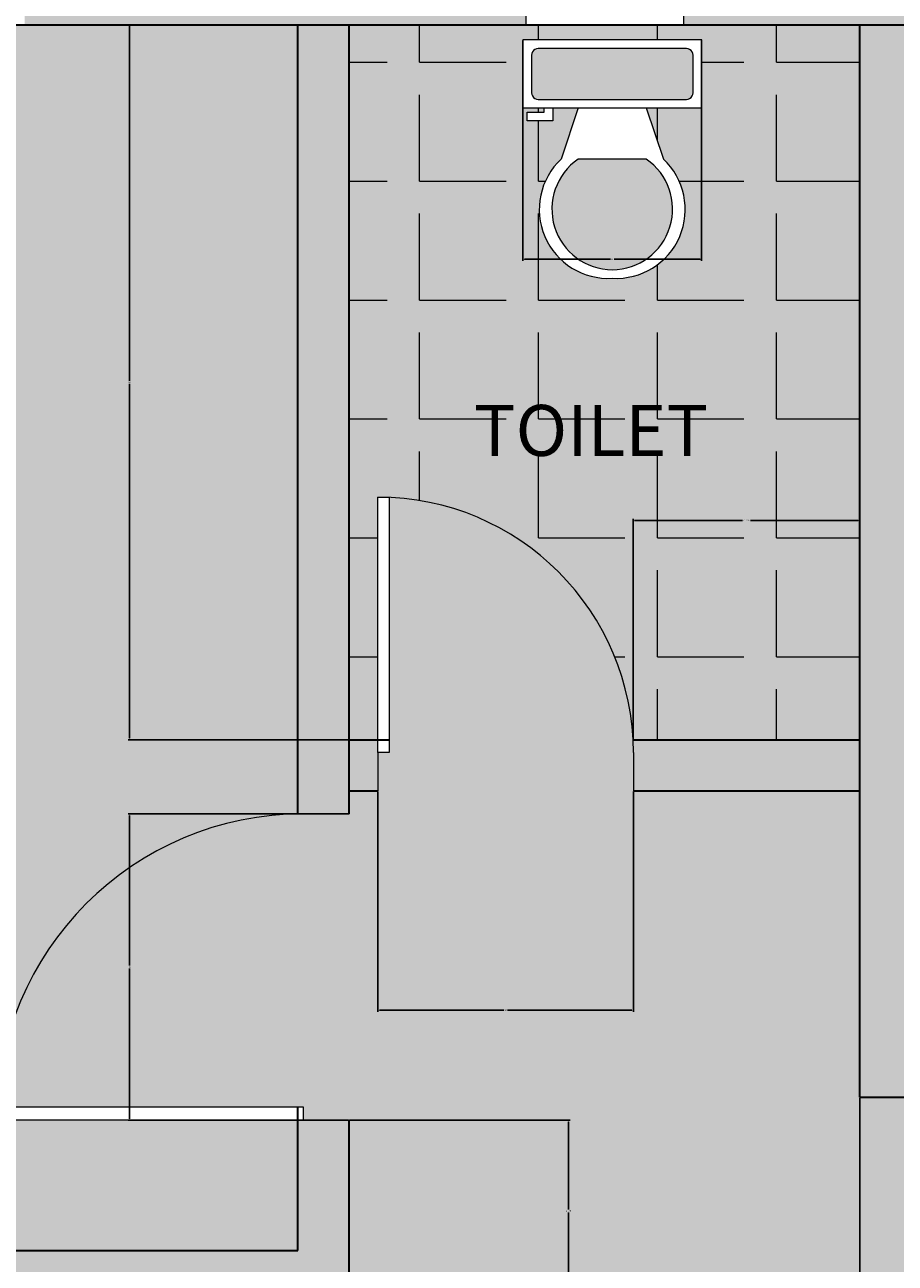
# Model space of a CAD drawing. Units: inches. Extents: x 3024 to 3952, y 1308 to 1863.
# Tile 23 of 29: x 3195 to 3297, y 1633 to 1779. Entities that reach past the tile are written whole.
import ezdxf

# ---------------------------------------------------------------- set-up
doc = ezdxf.new("R2010")
doc.units = ezdxf.units.IN
for name, color, linetype, lineweight in [('A-ANNO-DIMS', 2, 'Continuous', 18), ('A-AREA-IDEN', 7, 'Continuous', 18), ('A-DOOR', 4, 'Continuous', 18), ('A-FLOR-FIXT', 9, 'Continuous', 18), ('A-FLOR-FIXT-PATT', 7, 'Continuous', 13), ('A-FLOR-TILE-PATT', 7, 'Continuous', 13), ('A-GLAZ', 4, 'Continuous', 18), ('A-WALL', 7, 'Continuous', 35)]:
    doc.layers.add(name, color=color, linetype=linetype, lineweight=lineweight)
doc.layers.add('A-FLOR-PATT', color=254, linetype='Continuous', lineweight=13, true_color=0xfeeab9)
doc.layers.add('A-WALL-PATT', color=254, linetype='Continuous', lineweight=13, true_color=0xcecce6)
doc.styles.get("Standard").update_dxf_attribs({"font": 'arial.ttf'})
doc.dimstyles.get("Standard").update_dxf_attribs({"dimtxt": 0.18, "dimasz": 0.18, "dimexe": 0.18, "dimexo": 0.0625, "dimgap": 0.09, "dimtad": 0, "dimtih": 1, "dimtoh": 1, "dimdec": 4, "dimzin": 0, "dimdsep": 46, "dimtxsty": 'Standard', "dimcen": 0.09, "dimadec": 0, "dimazin": 0, "dimtfac": 1, "dimtdec": 4, "dimtofl": 0, "dimtmove": 0, "dimatfit": 3, "dimfxl": 1, "dimtolj": 1, "dimtzin": 0, "dimarcsym": 0})

# ---------------------------------------------------------------- blocks, each defined once
blk = doc.blocks.new('*U2')
for p, q in [((0, 0), (0, -6)), ((40, 0), (40, -6))]:
    blk.add_line(p, q)
blk.add_lwpolyline([(0, 0), (0, 40), (1.75, 40), (1.75, 0)], close=True)
blk.add_arc((0, 0), 40, 0, 90)
blk = doc.blocks.new('*U4')
for p, q in [((-40, 0), (-40, 6)), ((0, 0), (0, 6))]:
    blk.add_line(p, q)
blk.add_lwpolyline([(0, 0), (0, -40), (-1.75, -40), (-1.75, 0)], close=True)
blk.add_arc((0, 0), 40, 180, 270)
blk = doc.blocks.new('*U12')
for p, q in [((9.5, -6), (9.5, -2)), ((-10, -8.5), (-8, -8.5)), ((-10, -9.5), (-10, -8.5)), ((-8, -8.5), (-8, -8)), ((-7, -8), (-7, -9.5)), ((-4, -8), (-6, -14)), ((4, -8), (6, -14)), ((-7, -9.5), (-10, -9.5)), ((4, -14), (-4, -14))]:
    blk.add_line(p, q)
blk.add_lwpolyline([(10.5, -8), (10.5, 0), (-10.5, 0), (-10.5, -8)], close=True)
for points in [[(8.5, -1), (-8.5, -1)], [(-9.5, -2), (-9.5, -6)], [(-8.5, -7), (8.5, -7)]]:
    blk.add_lwpolyline(points)
for centre, radius, start, end in [((-8.625, -1.875), 0.8839, 81.8699, 188.1301), ((8.625, -1.875), 0.8839, 351.8699, 98.1301), ((-8.625, -6.125), 0.8839, 171.869898, 278.1301), ((8.625, -6.125), 0.8839, 261.8699, 8.1301), ((-0.4772, -19.9188), 8.0953, 133.01722, 273.38), ((0.0374, -19.8731), 7.127, 124.50543, 269.7), ((-0.0373, -19.8731), 7.127, 270.3, 55.4946), ((0.4773, -19.9188), 8.0953, 266.62, 46.9828)]:
    blk.add_arc(centre, radius, start, end)
blk = doc.blocks.new('WIN-BATH-18p5IN')
for p, q in [((0, 5.99), (0, 9)), ((18.52, 6.41), (18.52, 9)), ((18.52, 6.41), (18.52, 5.99)), ((0, 3.28), (0, 0)), ((18.52, 3.69), (18.52, 0))]:
    blk.add_line(p, q)
blk.add_lwpolyline([(0, 5.99), (18.52, 5.99), (18.52, 3.28), (0, 3.28)], close=True)
blk = doc.blocks.new('*D51')
at = {"layer": 'A-ANNO-DIMS', "color": 0, "lineweight": -2, "transparency": 16777216}
for p, q in [((3232.7, 1778.61), (3206.81, 1778.61)), ((3206.99, 1778.43), (3206.99, 1736.79)), ((3206.99, 1694.79), (3206.99, 1736.42)), ((3232.7, 1694.61), (3206.81, 1694.61))]:
    blk.add_line(p, q, dxfattribs=at)
at = {"layer": 'A-ANNO-DIMS', "color": 0, "transparency": 16777216}
for points in [[(3206.96, 1778.43), (3207.02, 1778.43), (3206.99, 1778.61)], [(3206.96, 1694.79), (3207.02, 1694.79), (3206.99, 1694.61)]]:
    blk.add_solid(points, dxfattribs=at)
at = {"layer": 'Defpoints', "color": 0, "transparency": 16777216}
for p in [(3206.99, 1778.61), (3232.76, 1778.61), (3232.76, 1694.61)]:
    blk.add_point(p, dxfattribs=at)
at = {"layer": 'A-ANNO-DIMS', "color": 0, "transparency": 16777216, "insert": (3206.99, 1736.61), "char_height": 0.18, "attachment_point": 5}
blk.add_mtext('\\A1;84', dxfattribs=at)
blk = doc.blocks.new('*D56')
at = {"layer": 'A-ANNO-DIMS', "color": 0, "lineweight": -2, "transparency": 16777216}
for p, q in [((3236.16, 1688.54), (3236.16, 1662.65)), ((3266.16, 1688.54), (3266.16, 1662.65)), ((3236.34, 1662.83), (3250.94, 1662.83)), ((3265.98, 1662.83), (3251.38, 1662.83))]:
    blk.add_line(p, q, dxfattribs=at)
at = {"layer": 'A-ANNO-DIMS', "color": 0, "transparency": 16777216}
for points in [[(3236.34, 1662.86), (3236.34, 1662.8), (3236.16, 1662.83)], [(3265.98, 1662.86), (3265.98, 1662.8), (3266.16, 1662.83)]]:
    blk.add_solid(points, dxfattribs=at)
at = {"layer": 'Defpoints', "color": 0, "transparency": 16777216}
for p in [(3236.16, 1688.61), (3266.16, 1688.61), (3236.16, 1662.83)]:
    blk.add_point(p, dxfattribs=at)
at = {"layer": 'A-ANNO-DIMS', "color": 0, "transparency": 16777216, "insert": (3251.16, 1662.83), "char_height": 0.18, "attachment_point": 5}
blk.add_mtext('\\A1;30', dxfattribs=at)
blk = doc.blocks.new('*D57')
at = {"layer": 'A-ANNO-DIMS', "color": 0, "lineweight": -2, "transparency": 16777216}
for p, q in [((3266.12, 1694.67), (3266.12, 1720.56)), ((3266.3, 1720.38), (3278.98, 1720.38)), ((3292.58, 1720.38), (3279.91, 1720.38)), ((3292.76, 1694.67), (3292.76, 1720.56))]:
    blk.add_line(p, q, dxfattribs=at)
at = {"layer": 'A-ANNO-DIMS', "color": 0, "transparency": 16777216}
for points in [[(3266.3, 1720.41), (3266.3, 1720.35), (3266.12, 1720.38)], [(3292.58, 1720.41), (3292.58, 1720.35), (3292.76, 1720.38)]]:
    blk.add_solid(points, dxfattribs=at)
at = {"layer": 'Defpoints', "color": 0, "transparency": 16777216}
for p in [(3292.76, 1720.38), (3266.12, 1694.61), (3292.76, 1694.61)]:
    blk.add_point(p, dxfattribs=at)
at = {"layer": 'A-ANNO-DIMS', "color": 0, "transparency": 16777216, "insert": (3279.44, 1720.38), "char_height": 0.18, "attachment_point": 5}
blk.add_mtext('\\A1;26.643', dxfattribs=at)
blk = doc.blocks.new('*D58')
at = {"layer": 'A-ANNO-DIMS', "color": 0, "lineweight": -2, "transparency": 16777216}
for p, q in [((3232.7, 1685.9), (3206.81, 1685.9)), ((3206.99, 1685.72), (3206.99, 1668.08)), ((3206.99, 1650.08), (3206.99, 1667.72)), ((3232.7, 1649.9), (3206.81, 1649.9))]:
    blk.add_line(p, q, dxfattribs=at)
at = {"layer": 'A-ANNO-DIMS', "color": 0, "transparency": 16777216}
for points in [[(3206.96, 1685.72), (3207.02, 1685.72), (3206.99, 1685.9)], [(3206.96, 1650.08), (3207.02, 1650.08), (3206.99, 1649.9)]]:
    blk.add_solid(points, dxfattribs=at)
at = {"layer": 'Defpoints', "color": 0, "transparency": 16777216}
for p in [(3206.99, 1685.9), (3232.76, 1685.9), (3232.76, 1649.9)]:
    blk.add_point(p, dxfattribs=at)
at = {"layer": 'A-ANNO-DIMS', "color": 0, "transparency": 16777216, "insert": (3206.99, 1667.9), "char_height": 0.18, "attachment_point": 5}
blk.add_mtext('\\A1;36', dxfattribs=at)
blk = doc.blocks.new('*D59')
at = {"layer": 'A-ANNO-DIMS', "color": 0, "lineweight": -2, "transparency": 16777216}
for p, q in [((3232.83, 1649.9), (3258.72, 1649.9)), ((3258.54, 1649.72), (3258.54, 1639.43)), ((3258.54, 1628.79), (3258.54, 1639.07)), ((3232.83, 1628.61), (3258.72, 1628.61))]:
    blk.add_line(p, q, dxfattribs=at)
at = {"layer": 'A-ANNO-DIMS', "color": 0, "transparency": 16777216}
for points in [[(3258.51, 1649.72), (3258.57, 1649.72), (3258.54, 1649.9)], [(3258.51, 1628.79), (3258.57, 1628.79), (3258.54, 1628.61)]]:
    blk.add_solid(points, dxfattribs=at)
at = {"layer": 'Defpoints', "color": 0, "transparency": 16777216}
for p in [(3232.76, 1649.9), (3232.76, 1628.61), (3258.54, 1628.61)]:
    blk.add_point(p, dxfattribs=at)
at = {"layer": 'A-ANNO-DIMS', "color": 0, "transparency": 16777216, "insert": (3258.54, 1639.25), "char_height": 0.18, "attachment_point": 5}
blk.add_mtext('\\A1;21.29', dxfattribs=at)
blk = doc.blocks.new('*D63')
at = {"layer": 'A-ANNO-DIMS', "color": 0, "lineweight": -2, "transparency": 16777216}
for p, q in [((3292.76, 1652.54), (3292.76, 1626.65)), ((3322.54, 1652.54), (3322.54, 1626.65)), ((3292.94, 1626.83), (3307.25, 1626.83)), ((3322.36, 1626.83), (3308.05, 1626.83))]:
    blk.add_line(p, q, dxfattribs=at)
at = {"layer": 'A-ANNO-DIMS', "color": 0, "transparency": 16777216}
for points in [[(3292.94, 1626.86), (3292.94, 1626.8), (3292.76, 1626.83)], [(3322.36, 1626.86), (3322.36, 1626.8), (3322.54, 1626.83)]]:
    blk.add_solid(points, dxfattribs=at)
at = {"layer": 'Defpoints', "color": 0, "transparency": 16777216}
for p in [(3292.76, 1652.61), (3322.54, 1652.61), (3292.76, 1626.83)]:
    blk.add_point(p, dxfattribs=at)
at = {"layer": 'A-ANNO-DIMS', "color": 0, "transparency": 16777216, "insert": (3307.65, 1626.83), "char_height": 0.18, "attachment_point": 5}
blk.add_mtext('\\A1;29.77', dxfattribs=at)
blk = doc.blocks.new('*D79')
at = {"layer": 'A-ANNO-DIMS', "color": 0, "lineweight": -2, "transparency": 16777216}
for p, q in [((3253.18, 1776.77), (3253.18, 1750.87)), ((3274.18, 1776.77), (3274.18, 1750.87)), ((3253.36, 1751.05), (3263.48, 1751.05)), ((3274, 1751.05), (3263.89, 1751.05))]:
    blk.add_line(p, q, dxfattribs=at)
at = {"layer": 'A-ANNO-DIMS', "color": 0, "transparency": 16777216}
for points in [[(3253.36, 1751.08), (3253.36, 1751.02), (3253.18, 1751.05)], [(3274, 1751.08), (3274, 1751.02), (3274.18, 1751.05)]]:
    blk.add_solid(points, dxfattribs=at)
at = {"layer": 'Defpoints', "color": 0, "transparency": 16777216}
for p in [(3253.18, 1776.83), (3274.18, 1776.83), (3253.18, 1751.05)]:
    blk.add_point(p, dxfattribs=at)
at = {"layer": 'A-ANNO-DIMS', "color": 0, "transparency": 16777216, "insert": (3263.68, 1751.05), "char_height": 0.18, "attachment_point": 5}
blk.add_mtext('\\A1;21', dxfattribs=at)

msp = doc.modelspace()

# ---------------------------------------------------------------- hatches: boundary and pattern name
at = {"layer": 'A-FLOR-FIXT-PATT'}
h = msp.add_hatch(color=256, dxfattribs=at)
h.dxf.hatch_style = 1
h.paths.add_polyline_path([(3267.6843, 1762.8281), (3259.6842, 1762.8281, 0.73453329), (3263.6843, 1749.8282, 0.73452973)])
h.paths.add_polyline_path([(3273.1842, 1774.8281, 0.50000012), (3272.1842, 1775.8281), (3255.1842, 1775.8281, 0.50000012), (3254.1842, 1774.8281), (3254.1842, 1770.8281, 0.50000012), (3255.1842, 1769.8281), (3272.1842, 1769.8281, 0.50000012), (3273.1842, 1770.8281)])
at = {"layer": 'A-FLOR-PATT', "transparency": 33554531}
h = msp.add_hatch(color=256, dxfattribs=at)
h.dxf.hatch_style = 1
h.paths.add_polyline_path([(3166.764, 1628.6064), (3106.764, 1628.6064), (3106.764, 1532.6064), (3133.066, 1532.6064, -0.38700389), (3161.716, 1561.0777), (3161.716, 1561.1064), (3163.0285, 1561.1064), (3163.0285, 1532.6064), (3166.764, 1532.6064)])
h.paths.add_polyline_path([(3123.904, 1600.7821), (3117.9039, 1602.7821), (3117.9039, 1599.7821), (3119.4039, 1599.7821), (3119.4039, 1596.7821), (3118.4039, 1596.7821), (3118.4039, 1598.7821), (3117.9039, 1598.7821), (3117.9039, 1596.2821), (3109.9039, 1596.2821), (3109.9039, 1617.2821), (3117.9039, 1617.2821), (3117.9039, 1610.7821), (3123.9038, 1612.7821, -0.70257121), (3137.9039, 1606.7822, -0.70256205)], flags=16)
h.paths.add_polyline_path([(3123.9039, 1602.7822), (3123.9039, 1610.7822, -0.73453329), (3136.9039, 1606.7822, -0.73452973)], flags=0)
h.paths.add_polyline_path([(3116.1539, 1597.2821), (3111.9039, 1597.2821, -0.41421356), (3110.9039, 1598.0321), (3110.9039, 1615.2821, -0.41421356), (3111.6539, 1616.2821), (3115.9039, 1616.2821, -0.41421356), (3116.9039, 1615.5321), (3116.9039, 1598.2821, -0.41421356)], flags=0)
h.paths.add_polyline_path([(3292.764, 1778.6064), (3232.764, 1778.6064), (3232.764, 1694.6064), (3236.1584, 1694.6064), (3236.1584, 1723.1064), (3237.4709, 1723.1064), (3237.4709, 1723.0777, -0.38700389), (3266.1209, 1694.6064), (3292.764, 1694.6064)])
h.paths.add_polyline_path([(3263.6843, 1748.8282, -0.70256205), (3257.6842, 1762.8281), (3259.6842, 1768.8281), (3256.6842, 1768.8281), (3256.6842, 1767.3281), (3253.6842, 1767.3281), (3253.6842, 1768.3281), (3255.6842, 1768.3281), (3255.6842, 1768.8281), (3253.1842, 1768.8281), (3253.1842, 1776.8281), (3274.1842, 1776.8281), (3274.1842, 1768.8281), (3267.6842, 1768.8281), (3269.6842, 1762.8282, -0.70257121)], flags=16)
h.paths.add_polyline_path([(3263.6842, 1749.8282, -0.73452973), (3259.6842, 1762.8281), (3267.6843, 1762.8281, -0.73453329)], flags=0)
h.paths.add_polyline_path([(3255.1842, 1769.8281, -0.41421356), (3254.1842, 1770.5781), (3254.1842, 1774.8281, -0.41421356), (3254.9342, 1775.8281), (3272.1842, 1775.8281, -0.41421356), (3273.1842, 1775.0781), (3273.1842, 1770.8281, -0.41421356), (3272.4342, 1769.8281)], flags=0)
h.paths.add_polyline_path([(3460.764, 1778.6064), (3412.764, 1778.6064), (3412.764, 1745.5689, -0.38700389), (3441.2353, 1716.9189), (3441.264, 1716.9189), (3441.264, 1715.6064), (3412.764, 1715.6064), (3412.764, 1694.6064), (3460.764, 1694.6064)])
h.paths.add_polyline_path([(3121.3033, 1577.378), (3153.693, 1577.378), (3153.693, 1586.6752), (3121.3033, 1586.6752)], flags=24)
h.paths.add_polyline_path([(3245.8895, 1726.2997), (3278.2793, 1726.2997), (3278.2793, 1735.5968), (3245.8895, 1735.5968)], flags=24)
h.paths.add_polyline_path([(3419.204, 1753.8578), (3453.3997, 1753.8578), (3453.3997, 1762.9956), (3419.204, 1762.9956)], flags=24)
at = {"layer": 'A-FLOR-PATT', "transparency": 33554528}
h = msp.add_hatch(color=256, dxfattribs=at)
h.dxf.hatch_style = 1
h.paths.add_polyline_path([(3460.764, 1688.6064), (3412.764, 1688.6064), (3412.764, 1694.6064), (3460.764, 1694.6064), (3460.764, 1778.6064), (3406.764, 1778.6064), (3406.764, 1759.9514), (3318.2981, 1759.9514), (3318.2981, 1658.6064), (3322.5356, 1658.6064), (3322.5356, 1652.6064), (3292.764, 1652.6064), (3292.764, 1778.6064), (3106.764, 1778.6064), (3106.764, 1628.6064), (3172.764, 1628.6064), (3172.764, 1532.6064), (3166.764, 1532.6064), (3166.764, 1628.6064), (3106.764, 1628.6064), (3106.764, 1356.8452), (3202.812, 1356.8452), (3202.812, 1354.2534), (3202.812, 1353.8388), (3202.812, 1351.1212), (3202.812, 1347.8452), (3277.764, 1347.8452), (3277.764, 1353.8452), (3277.764, 1356.8452), (3277.764, 1442.6064), (3460.764, 1442.6064)])
h.paths.add_polyline_path([(3216.238, 1527.2064), (3216.238, 1491.2064), (3214.663, 1491.2064), (3214.663, 1491.2409, -0.39662236), (3180.243, 1526.6064), (3163.0285, 1526.6064), (3163.0285, 1531.1064), (3161.716, 1531.1064), (3161.716, 1561.1064), (3163.0285, 1561.1064), (3163.0285, 1531.1064), (3163.0285, 1526.6064), (3180.243, 1526.6064, 0.39662236), (3214.663, 1491.2409), (3214.663, 1527.2064)], flags=16)
h.paths.add_polyline_path([(3227.364, 1649.8972), (3191.364, 1649.8972), (3191.364, 1651.4722), (3227.364, 1651.4722)], flags=16)
h.paths.add_polyline_path([(3323.1172, 1606.7362), (3323.8545, 1606.8514), (3323.8545, 1594.8241), (3323.1172, 1594.9393)], flags=16)
h.paths.add_polyline_path([(3324.2232, 1606.909), (3330.1216, 1607.8307), (3330.1216, 1614.1093), (3339.3495, 1614.1093), (3340.2711, 1620.0078), (3352.4136, 1620.0078), (3353.3353, 1614.1093), (3359.9941, 1614.1093), (3360.9157, 1620.0078), (3373.0582, 1620.0078), (3373.9799, 1614.1093), (3383.2077, 1614.1093), (3383.2077, 1607.8307), (3389.1062, 1606.909), (3389.1062, 1594.7665), (3383.2077, 1593.8449), (3383.2077, 1587.5663), (3373.9799, 1587.5663), (3373.0583, 1581.6678), (3360.9157, 1581.6678), (3359.9941, 1587.5663), (3353.3353, 1587.5663), (3352.4136, 1581.6678), (3340.2711, 1581.6678), (3339.3495, 1587.5663), (3330.1216, 1587.5663), (3330.1216, 1593.8449), (3324.2232, 1594.7665)], flags=16)
h.paths.add_polyline_path([(3236.1584, 1693.1064), (3236.1584, 1723.1064), (3237.4709, 1723.1064), (3237.4709, 1693.1064)], flags=16)
h.paths.add_polyline_path([(3373.2158, 1600.6847), (3373.7965, 1600.7303), (3374.3268, 1600.7874), (3374.8132, 1600.8531), (3375.2621, 1600.9247), (3375.6801, 1600.9991), (3376.0736, 1601.0735), (3376.6855, 1601.19), (3377.366, 1601.3023), (3378.0667, 1601.3814), (3378.8026, 1601.4123), (3379.5865, 1601.3839), (3380.4537, 1601.2948), (3381.301, 1601.1717), (3382.0317, 1601.0433), (3382.4398, 1600.9607), (3382.6252, 1600.9201), (3382.919, 1600.8507), (3382.9044, 1600.8531), (3382.842, 1600.8678), (3382.7541, 1600.8896), (3382.6252, 1600.9201), (3382.4398, 1600.9607), (3382.1868, 1601.0119), (3381.8738, 1601.0711), (3381.5125, 1601.1346), (3381.1149, 1601.1988), (3380.6928, 1601.2601), (3380.2581, 1601.3149), (3379.8226, 1601.3597), (3379.3984, 1601.3908), (3378.9944, 1601.4054), (3378.6092, 1601.4042), (3378.2384, 1601.3886), (3377.8777, 1601.36), (3377.5227, 1601.32), (3377.1691, 1601.2698), (3376.8127, 1601.211), (3376.4491, 1601.145), (3376.0736, 1601.0735), (3375.4177, 1600.9494), (3374.5542, 1600.8119), (3373.5044, 1600.6988)], flags=0)
h.paths.add_polyline_path([(3380.0253, 1596.7351), (3380.499, 1596.6659), (3380.9706, 1596.6119), (3381.4375, 1596.5791), (3381.8971, 1596.5736), (3382.5886, 1596.6167), (3382.7848, 1596.6692), (3382.1465, 1596.5706), (3381.236, 1596.5815), (3380.3199, 1596.6865)], flags=0)
h.paths.add_polyline_path([(3369.6414, 1603.9617), (3370.1589, 1604.0021), (3370.6218, 1604.0539), (3371.0335, 1604.1173), (3371.3978, 1604.1921), (3371.7181, 1604.2785), (3371.9984, 1604.3761), (3372.2441, 1604.483), (3372.4611, 1604.5972), (3372.655, 1604.7163), (3372.8317, 1604.8384), (3372.9968, 1604.9611), (3373.3703, 1605.2455), (3373.8426, 1605.5328), (3374.4624, 1605.7539), (3375.1058, 1605.8302), (3375.7221, 1605.8261), (3376.4109, 1605.76), (3377.1534, 1605.6376), (3377.8945, 1605.473), (3378.1382, 1605.409), (3377.7394, 1605.5074), (3377.3509, 1605.5937), (3376.9704, 1605.6677), (3376.5999, 1605.7288), (3376.2417, 1605.7762), (3375.8979, 1605.8092), (3375.5707, 1605.8271), (3375.2621, 1605.8291), (3374.9745, 1605.8146), (3374.7092, 1605.7832), (3374.4647, 1605.7359), (3374.239, 1605.6742), (3374.0298, 1605.5996), (3373.835, 1605.5134), (3373.6525, 1605.4171), (3373.4801, 1605.3123), (3373.3156, 1605.2002), (3373.1562, 1605.0825), (3372.7603, 1604.781), (3372.236, 1604.4588), (3371.5738, 1604.2283), (3370.8493, 1604.0794), (3369.9262, 1603.976)], flags=0)
h.paths.add_polyline_path([(3366.7533, 1606.5832), (3367.1713, 1606.5519), (3367.5378, 1606.5374), (3367.8568, 1606.5394), (3368.1325, 1606.5573), (3368.3694, 1606.5903), (3368.5717, 1606.6377), (3368.7438, 1606.6988), (3368.89, 1606.7728), (3369.0146, 1606.8591), (3369.121, 1606.9568), (3369.2094, 1607.0646), (3369.2792, 1607.181), (3369.3295, 1607.3046), (3369.3596, 1607.4339), (3369.3688, 1607.5676), (3369.3565, 1607.7042), (3369.3218, 1607.8422), (3369.2649, 1607.9804), (3369.1893, 1608.1187), (3369.0993, 1608.2569), (3368.9992, 1608.3952), (3368.8934, 1608.5334), (3368.7861, 1608.6717), (3368.6817, 1608.8099), (3368.4212, 1609.1804), (3368.2685, 1609.7106), (3368.4883, 1610.1814), (3369.0537, 1610.4604), (3369.6717, 1610.5097), (3370.2812, 1610.3612), (3370.4805, 1610.2968), (3370.1882, 1610.3839), (3369.9284, 1610.4472), (3369.6905, 1610.4842), (3369.4662, 1610.4933), (3369.2555, 1610.4765), (3369.0608, 1610.4367), (3368.884, 1610.3767), (3368.7274, 1610.2994), (3368.5931, 1610.2077), (3368.4833, 1610.1045), (3368.4002, 1609.9927), (3368.3451, 1609.8747), (3368.3166, 1609.7517), (3368.3127, 1609.6244), (3368.331, 1609.4935), (3368.3696, 1609.3597), (3368.4261, 1609.2237), (3368.4985, 1609.0863), (3368.5845, 1608.9482), (3368.6817, 1608.8099), (3368.7861, 1608.6717), (3368.8934, 1608.5334), (3368.9992, 1608.3952), (3369.0993, 1608.2569), (3369.3398, 1607.8876), (3369.3941, 1607.2896), (3368.9774, 1606.7817), (3368.3928, 1606.5742), (3367.7162, 1606.5303), (3367.0044, 1606.5585)], flags=0)
h.paths.add_polyline_path([(3362.1859, 1610.2589), (3362.5478, 1610.2845), (3362.8348, 1610.3275), (3363.0585, 1610.3863), (3363.2303, 1610.4595), (3363.3619, 1610.5457), (3363.463, 1610.6432), (3363.5376, 1610.7502), (3363.5876, 1610.8643), (3363.6153, 1610.9834), (3363.6229, 1611.1055), (3363.6125, 1611.2283), (3363.5861, 1611.3496), (3363.5462, 1611.4673), (3363.4949, 1611.5797), (3363.4358, 1611.6871), (3363.3723, 1611.7902), (3363.3081, 1611.8897), (3363.2468, 1611.9863), (3363.192, 1612.0808), (3363.0258, 1612.4261), (3363.3371, 1612.8672), (3363.9008, 1612.9782), (3364.4822, 1612.9641), (3365.1098, 1612.9074), (3365.328, 1612.8805), (3364.9615, 1612.9208), (3364.6426, 1612.9496), (3364.3668, 1612.9669), (3364.1299, 1612.9726), (3363.9276, 1612.9669), (3363.7555, 1612.9496), (3363.6093, 1612.9208), (3363.4848, 1612.8805), (3363.3782, 1612.8289), (3363.2889, 1612.7672), (3363.2169, 1612.6969), (3363.1622, 1612.6193), (3363.1247, 1612.5361), (3363.1046, 1612.4484), (3363.1017, 1612.358), (3363.1161, 1612.266), (3363.1472, 1612.1738), (3363.192, 1612.0808), (3363.2468, 1611.9863), (3363.3081, 1611.8897), (3363.3723, 1611.7902), (3363.4358, 1611.6871), (3363.6363, 1611.323), (3363.5979, 1610.7003), (3363.0863, 1610.3651), (3362.3983, 1610.2622)], flags=0)
h.paths.add_polyline_path([(3352.356, 1581.2991), (3352.2408, 1580.5618), (3340.4439, 1580.5618), (3340.3287, 1581.2991)], flags=16)
h.paths.add_polyline_path([(3340.4439, 1621.1137), (3352.2408, 1621.1137), (3352.356, 1620.3764), (3340.3287, 1620.3764)], flags=16)
h.paths.add_polyline_path([(3278.4282, 1504.7424), (3290.3831, 1504.7424), (3290.3831, 1502.7499), (3291.0473, 1502.7499), (3291.0473, 1494.7799), (3290.3831, 1494.7799), (3290.3831, 1494.1158), (3291.0473, 1494.1158), (3291.0473, 1486.1458), (3290.3831, 1486.1458), (3290.3831, 1484.1533), (3291.0473, 1484.1533), (3291.0473, 1483.4892, -0.09090909), (3291.0473, 1468.8776), (3291.0473, 1468.2135), (3290.3831, 1468.2135), (3290.3831, 1464.8926), (3278.4282, 1464.8926), (3278.4282, 1472.8626), (3277.764, 1473.5268), (3277.764, 1478.84), (3278.4282, 1479.5042)], flags=16)
h.paths.add_polyline_path([(3278.7603, 1504.4103), (3290.051, 1504.4103), (3290.051, 1465.2247), (3278.7603, 1465.2247)], flags=0)
h.paths.add_polyline_path([(3123.904, 1600.7821), (3117.9039, 1602.7821), (3117.9039, 1599.7821), (3119.4039, 1599.7821), (3119.4039, 1596.7821), (3118.4039, 1596.7821), (3118.4039, 1598.7821), (3117.9039, 1598.7821), (3117.9039, 1596.2821), (3109.9039, 1596.2821), (3109.9039, 1617.2821), (3117.9039, 1617.2821), (3117.9039, 1610.7821), (3123.9038, 1612.7821, -0.70257121), (3137.9039, 1606.7822, -0.70256205)], flags=16)
h.paths.add_polyline_path([(3123.9039, 1602.7822), (3123.9039, 1610.7822, -0.73453329), (3136.9039, 1606.7822, -0.73452973)], flags=0)
h.paths.add_polyline_path([(3177.972, 1689.6473), (3109.2405, 1689.6473), (3109.2405, 1741.1959), (3177.972, 1741.1959)], flags=16)
h.paths.add_polyline_path([(3373.0006, 1581.2991), (3372.8854, 1580.5618), (3361.0885, 1580.5618), (3360.9733, 1581.2991)], flags=16)
h.paths.add_polyline_path([(3361.0885, 1621.1137), (3372.8854, 1621.1137), (3373.0006, 1620.3764), (3360.9733, 1620.3764)], flags=16)
h.paths.add_polyline_path([(3116.9039, 1598.2821, -0.41421356), (3116.1539, 1597.2821), (3111.9039, 1597.2821, -0.41421356), (3110.9039, 1598.0321), (3110.9039, 1615.2821, -0.41421356), (3111.6539, 1616.2821), (3115.9039, 1616.2821, -0.41421356), (3116.9039, 1615.5321)], flags=0)
h.paths.add_polyline_path([(3121.6122, 1728.1369), (3121.6122, 1696.5205), (3110.2715, 1696.5205), (3110.2715, 1714.3906), (3121.6122, 1714.3906), (3121.6122, 1716.4526), (3110.2715, 1716.4526), (3110.2715, 1734.3228), (3123.3304, 1734.3228), (3123.3304, 1729.8552), (3134.6711, 1741.1959), (3134.6711, 1728.1369)], flags=0)
h.paths.add_polyline_path([(3389.4748, 1606.8514), (3390.2122, 1606.7362), (3390.2122, 1594.9393), (3389.4748, 1594.8241)], flags=16)
h.paths.add_polyline_path([(3257.6842, 1762.8281), (3259.6842, 1768.8281), (3256.6842, 1768.8281), (3256.6842, 1767.3281), (3253.6842, 1767.3281), (3253.6842, 1768.3281), (3255.6842, 1768.3281), (3255.6842, 1768.8281), (3253.1842, 1768.8281), (3253.1842, 1776.8281), (3274.1842, 1776.8281), (3274.1842, 1768.8281), (3267.6842, 1768.8281), (3269.6842, 1762.8282, -0.70257121), (3263.6843, 1748.8282, -0.70256205)], flags=16)
h.paths.add_polyline_path([(3259.6842, 1762.8281), (3267.6843, 1762.8281, -0.73453329), (3263.6842, 1749.8282, -0.73452973)], flags=0)
h.paths.add_polyline_path([(3411.264, 1715.6064), (3411.264, 1716.9189), (3441.264, 1716.9189), (3441.264, 1715.6064)], flags=16)
h.paths.add_polyline_path([(3178.3806, 1449.1876), (3178.3806, 1397.639), (3109.6491, 1397.639), (3109.6491, 1449.1876)], flags=16)
h.paths.add_polyline_path([(3397.1501, 1541.7146), (3419.6183, 1541.7146), (3419.6183, 1496.7783), (3397.1501, 1496.7783)], flags=16)
h.paths.add_polyline_path([(3254.1842, 1770.5781), (3254.1842, 1774.8281, -0.41421356), (3254.9342, 1775.8281), (3272.1842, 1775.8281, -0.41421356), (3273.1842, 1775.0781), (3273.1842, 1770.8281, -0.41421356), (3272.4342, 1769.8281), (3255.1842, 1769.8281, -0.41421356)], flags=0)
h.paths.add_polyline_path([(3403.672, 1500.7601), (3403.6016, 1500.3997), (3403.5328, 1500.0441), (3403.4662, 1499.6867), (3403.4027, 1499.3226), (3403.3464, 1498.9532), (3403.3025, 1498.5811), (3403.2759, 1498.2091), (3403.2714, 1497.8401), (3403.3064, 1497.2813), (3403.3491, 1497.1219), (3403.2689, 1497.6395), (3403.2778, 1498.3719), (3403.3635, 1499.0984), (3403.4889, 1499.8168), (3403.6016, 1500.3997), (3403.672, 1500.7601), (3403.744, 1501.1315), (3403.817, 1501.5205), (3403.891, 1501.9336), (3403.9656, 1502.3769), (3404.0404, 1502.8572), (3404.115, 1503.3786), (3404.2264, 1504.2311), (3404.2571, 1504.5223), (3404.1552, 1503.6598), (3404.0063, 1502.6193), (3403.8604, 1501.7518), (3403.744, 1501.1315)], flags=0)
h.paths.add_polyline_path([(3406.5868, 1505.0416), (3406.6121, 1504.5236), (3406.6492, 1504.0526), (3406.6956, 1503.624), (3406.7491, 1503.2333), (3406.8072, 1502.8759), (3406.8676, 1502.5473), (3406.9281, 1502.243), (3407.0268, 1501.7597), (3407.1416, 1501.1368), (3407.2087, 1500.3904), (3407.1804, 1499.6703), (3407.1078, 1498.9956), (3407.0074, 1498.3199), (3406.8809, 1497.6059), (3406.7403, 1496.9627), (3406.7418, 1496.9824), (3406.7491, 1497.0249), (3406.8229, 1497.3409), (3406.8364, 1497.4025), (3406.878, 1497.6078), (3406.9261, 1497.8614), (3406.9777, 1498.1526), (3407.0298, 1498.4712), (3407.0797, 1498.8068), (3407.1243, 1499.149), (3407.1607, 1499.4874), (3407.1859, 1499.8115), (3407.1978, 1500.1137), (3407.1969, 1500.3962), (3407.1841, 1500.6642), (3407.1609, 1500.9225), (3407.1284, 1501.1761), (3407.0876, 1501.43), (3407.0398, 1501.6891), (3406.9862, 1501.9585), (3406.8832, 1502.4628), (3406.7712, 1503.0713), (3406.6657, 1503.8424), (3406.5924, 1504.7735)], flags=0)
h.paths.add_polyline_path([(3409.2517, 1507.8962), (3409.2752, 1507.4282), (3409.3079, 1507.0076), (3409.3501, 1506.6314), (3409.4015, 1506.2969), (3409.4624, 1506.0009), (3409.5326, 1505.7406), (3409.6119, 1505.5128), (3409.6988, 1505.3131), (3409.7915, 1505.1368), (3409.8883, 1504.9792), (3409.9875, 1504.8356), (3410.0872, 1504.7015), (3410.1859, 1504.572), (3410.4508, 1504.2132), (3410.7205, 1503.6035), (3410.8059, 1502.8824), (3410.7619, 1502.0875), (3410.6122, 1501.2299), (3410.4402, 1500.6169), (3410.2538, 1500.0031), (3410.0536, 1499.3219), (3409.9909, 1499.0812), (3410.1761, 1499.7472), (3410.3596, 1500.3513), (3410.4512, 1500.6561), (3410.5312, 1500.9412), (3410.6013, 1501.226), (3410.6614, 1501.512), (3410.7111, 1501.7964), (3410.7496, 1502.0763), (3410.7764, 1502.3489), (3410.7909, 1502.6114), (3410.7926, 1502.8608), (3410.7808, 1503.0944), (3410.7553, 1503.31), (3410.7169, 1503.5087), (3410.6667, 1503.6921), (3410.6061, 1503.8621), (3410.5361, 1504.0203), (3410.4578, 1504.1686), (3410.3726, 1504.3088), (3410.2815, 1504.4424), (3410.1859, 1504.572), (3410.0872, 1504.7015), (3409.859, 1505.0083), (3409.5943, 1505.5117), (3409.4266, 1506.1336), (3409.324, 1506.8011), (3409.2586, 1507.6407)], flags=0)
h.paths.add_polyline_path([(3411.4914, 1510.5878), (3411.4432, 1510.1586), (3411.4054, 1509.775), (3411.38, 1509.4354), (3411.3681, 1509.1376), (3411.3698, 1508.8784), (3411.3843, 1508.6542), (3411.4112, 1508.4618), (3411.4497, 1508.2974), (3411.4994, 1508.1575), (3411.5595, 1508.0388), (3411.6296, 1507.9375), (3411.7097, 1507.851), (3411.802, 1507.7792), (3411.9096, 1507.7225), (3412.0353, 1507.6817), (3412.1821, 1507.6572), (3412.3528, 1507.6496), (3412.5505, 1507.6597), (3412.778, 1507.6879), (3413.0364, 1507.7341), (3413.3194, 1507.7955), (3413.6188, 1507.8687), (3413.9264, 1507.95), (3414.234, 1508.036), (3414.5333, 1508.1232), (3414.8163, 1508.208), (3415.0747, 1508.287), (3415.3023, 1508.3569), (3415.5007, 1508.4158), (3415.6733, 1508.4617), (3416.1158, 1508.5538), (3416.512, 1508.2591), (3416.716, 1507.6581), (3416.61, 1507.0003), (3416.3052, 1506.3411), (3415.8928, 1505.618), (3415.7339, 1505.3633), (3415.9914, 1505.791), (3416.201, 1506.1583), (3416.3666, 1506.4739), (3416.4925, 1506.7462), (3416.5828, 1506.9838), (3416.6413, 1507.1949), (3416.6725, 1507.3883), (3416.6799, 1507.5705), (3416.6662, 1507.7417), (3416.6339, 1507.9), (3416.5851, 1508.0436), (3416.5223, 1508.1709), (3416.4478, 1508.28), (3416.3639, 1508.3692), (3416.273, 1508.4368), (3416.1765, 1508.4815), (3416.0718, 1508.5047), (3415.9553, 1508.5079), (3415.8237, 1508.493), (3415.6733, 1508.4617), (3415.5007, 1508.4158), (3415.3327, 1508.3659), (3414.6495, 1508.157), (3414.0606, 1507.9855), (3413.4456, 1507.8229), (3412.8838, 1507.701), (3412.5505, 1507.6597), (3412.0748, 1507.6354), (3411.595, 1507.8883), (3411.398, 1508.4429), (3411.3624, 1508.9927), (3411.3854, 1509.5711), (3411.4578, 1510.3071)], flags=0)
h.paths.add_polyline_path([(3135.0797, 1449.1876), (3135.0797, 1436.1286), (3122.0208, 1436.1286), (3122.0208, 1404.5122), (3110.6801, 1404.5122), (3110.6801, 1422.3823), (3122.0208, 1422.3823), (3122.0208, 1424.4443), (3110.6801, 1424.4443), (3110.6801, 1442.3145), (3123.739, 1442.3145), (3123.739, 1437.8469)], flags=0)
h.paths.add_polyline_path([(3416.4944, 1514.2949), (3416.4837, 1513.8511), (3416.4893, 1513.4867), (3416.5102, 1513.1926), (3416.5451, 1512.9593), (3416.5929, 1512.7775), (3416.6524, 1512.6379), (3416.7224, 1512.531), (3416.8017, 1512.4488), (3416.8886, 1512.3882), (3416.9813, 1512.3476), (3417.0781, 1512.3251), (3417.1773, 1512.3189), (3417.277, 1512.3274), (3417.3757, 1512.3488), (3417.4713, 1512.3813), (3417.5627, 1512.4229), (3417.65, 1512.471), (3417.7338, 1512.5225), (3417.8146, 1512.5747), (3417.8931, 1512.6245), (3417.9699, 1512.6691), (3418.2968, 1512.8265), (3418.6505, 1512.4645), (3418.7037, 1511.9342), (3418.6693, 1511.3839), (3418.6076, 1510.8228), (3418.5777, 1510.5927), (3418.6197, 1510.9333), (3418.6525, 1511.2311), (3418.6759, 1511.4903), (3418.6899, 1511.7144), (3418.6946, 1511.9069), (3418.6899, 1512.0713), (3418.6759, 1512.2112), (3418.6525, 1512.33), (3418.6197, 1512.4311), (3418.5778, 1512.5177), (3418.5276, 1512.5903), (3418.4705, 1512.6488), (3418.4075, 1512.6933), (3418.3399, 1512.7237), (3418.2686, 1512.7401), (3418.1951, 1512.7424), (3418.1204, 1512.7307), (3418.0455, 1512.7055), (3417.9792, 1512.6736), (3417.65, 1512.471), (3417.5627, 1512.4229), (3417.4713, 1512.3813), (3417.3757, 1512.3488), (3417.277, 1512.3274), (3416.878, 1512.2936), (3416.5757, 1512.7549), (3416.492, 1513.3145), (3416.4808, 1514.0384)], flags=0)
h.paths.add_polyline_path([(3392.8223, 1481.9454), (3396.7707, 1481.9454), (3396.7707, 1480.9201), (3428.3585, 1480.9201), (3428.3585, 1481.9454), (3432.3069, 1481.9454), (3432.3069, 1464.8354, -0.26666697), (3392.8223, 1464.8354)], flags=16)
h.paths.add_polyline_path([(3431.203, 1547.5428), (3450.8613, 1547.5428, -0.19047621), (3450.8614, 1484.031), (3431.203, 1484.031), (3431.203, 1488.5675), (3432.3809, 1488.5675), (3432.3809, 1543.0062), (3431.203, 1543.0062)], flags=16)
h.paths.add_polyline_path([(3451.9233, 1524.86, -0.04962821), (3451.9233, 1506.7138), (3446.7921, 1506.7138), (3446.7921, 1524.86)], flags=0)
h.paths.add_polyline_path([(3460.764, 1436.6064), (3277.764, 1436.6064), (3277.764, 1356.8452), (3277.764, 1353.8452), (3460.764, 1353.8452)], flags=17)
h.paths.add_polyline_path([(3121.3033, 1577.378), (3153.693, 1577.378), (3153.693, 1586.6752), (3121.3033, 1586.6752)], flags=24)
h.paths.add_polyline_path([(3164.1457, 1464.1276), (3210.4801, 1464.1276), (3210.4801, 1473.4247), (3164.1457, 1473.4247)], flags=24)
h.paths.add_polyline_path([(3343.1909, 1505.8863), (3373.7236, 1505.8863), (3373.7236, 1515.1773), (3343.1909, 1515.1773)], flags=24)
h.paths.add_polyline_path([(3337.6353, 1564.2926), (3370.0189, 1564.2926), (3370.0189, 1573.5836), (3337.6353, 1573.5836)], flags=24)
h.paths.add_polyline_path([(3419.204, 1753.8578), (3453.3997, 1753.8578), (3453.3997, 1762.9956), (3419.204, 1762.9956)], flags=24)
h.paths.add_polyline_path([(3341.2523, 1701.0246), (3381.0761, 1701.0246), (3381.0761, 1710.3156), (3341.2523, 1710.3156)], flags=24)
h.paths.add_polyline_path([(3245.8895, 1726.2997), (3278.2793, 1726.2997), (3278.2793, 1735.5968), (3245.8895, 1735.5968)], flags=24)
h.paths.add_polyline_path([(3128.8045, 1668.6736), (3175.1389, 1668.6736), (3175.1389, 1677.9707), (3128.8045, 1677.9707)], flags=24)
h.paths.add_polyline_path([(3345.9997, 1396.0062), (3389.09, 1396.0062), (3389.09, 1405.3033), (3345.9997, 1405.3033)], flags=24)
at = {"layer": 'A-FLOR-TILE-PATT', "transparency": 33554569}
h = msp.add_hatch(dxfattribs=at)
h.set_pattern_fill('ANGLE', color=256, scale=2)
h.set_pattern_definition([(0, (0, 0), (0, 13.97), [10.16, -3.81]), (90, (0, 0), (-13.97, 9e-16), [10.16, -3.81])])
h.paths.add_polyline_path([(3292.764, 1778.6064), (3232.764, 1778.6064), (3232.764, 1694.6064), (3236.1584, 1694.6064), (3236.1584, 1723.1064), (3237.4709, 1723.1064), (3237.4709, 1723.0777, -0.38700389), (3266.1209, 1694.6064), (3292.764, 1694.6064)])
h.paths.add_polyline_path([(3263.6843, 1748.8282, -0.70256205), (3257.6842, 1762.8281), (3259.6842, 1768.8281), (3256.6842, 1768.8281), (3256.6842, 1767.3281), (3253.6842, 1767.3281), (3253.6842, 1768.3281), (3255.6842, 1768.3281), (3255.6842, 1768.8281), (3253.1842, 1768.8281), (3253.1842, 1776.8281), (3274.1842, 1776.8281), (3274.1842, 1768.8281), (3267.6842, 1768.8281), (3269.6842, 1762.8282, -0.70257121)], flags=16)
h.paths.add_polyline_path([(3263.6842, 1749.8282, -0.73452973), (3259.6842, 1762.8281), (3267.6843, 1762.8281, -0.73453329)], flags=0)
h.paths.add_polyline_path([(3255.1842, 1769.8281, -0.41421356), (3254.1842, 1770.5781), (3254.1842, 1774.8281, -0.41421356), (3254.9342, 1775.8281), (3272.1842, 1775.8281, -0.41421356), (3273.1842, 1775.0781), (3273.1842, 1770.8281, -0.41421356), (3272.4342, 1769.8281)], flags=0)
h.paths.add_polyline_path([(3460.764, 1436.6064), (3277.764, 1436.6064), (3277.764, 1356.8452), (3277.764, 1353.8452), (3460.764, 1353.8452)])
h.paths.add_polyline_path([(3166.764, 1628.6064), (3106.764, 1628.6064), (3106.764, 1532.6064), (3133.066, 1532.6064, -0.38700389), (3161.716, 1561.0777), (3161.716, 1561.1064), (3163.0285, 1561.1064), (3163.0285, 1532.6064), (3166.764, 1532.6064)])
h.paths.add_polyline_path([(3123.904, 1600.7821), (3117.9039, 1602.7821), (3117.9039, 1599.7821), (3119.4039, 1599.7821), (3119.4039, 1596.7821), (3118.4039, 1596.7821), (3118.4039, 1598.7821), (3117.9039, 1598.7821), (3117.9039, 1596.2821), (3109.9039, 1596.2821), (3109.9039, 1617.2821), (3117.9039, 1617.2821), (3117.9039, 1610.7821), (3123.9038, 1612.7821, -0.70257121), (3137.9039, 1606.7822, -0.70256205)], flags=16)
h.paths.add_polyline_path([(3123.9039, 1602.7822), (3123.9039, 1610.7822, -0.73453329), (3136.9039, 1606.7822, -0.73452973)], flags=0)
h.paths.add_polyline_path([(3116.1539, 1597.2821), (3111.9039, 1597.2821, -0.41421356), (3110.9039, 1598.0321), (3110.9039, 1615.2821, -0.41421356), (3111.6539, 1616.2821), (3115.9039, 1616.2821, -0.41421356), (3116.9039, 1615.5321), (3116.9039, 1598.2821, -0.41421356)], flags=0)
h.paths.add_polyline_path([(3245.8895, 1726.2997), (3278.2793, 1726.2997), (3278.2793, 1735.5968), (3245.8895, 1735.5968)], flags=24)
h.paths.add_polyline_path([(3345.9997, 1396.0062), (3389.09, 1396.0062), (3389.09, 1405.3033), (3345.9997, 1405.3033)], flags=24)
h.paths.add_polyline_path([(3121.3033, 1577.378), (3153.693, 1577.378), (3153.693, 1586.6752), (3121.3033, 1586.6752)], flags=24)
at = {"layer": 'A-WALL-PATT'}
h = msp.add_hatch(color=256, dxfattribs=at)
h.dxf.hatch_style = 1
h.paths.add_polyline_path([(3106.764, 1778.6064), (3140.5977, 1778.6064), (3140.5977, 1781.8824), (3140.5977, 1784.6), (3140.5977, 1787.6064), (3097.764, 1787.6064), (3097.764, 1590.213), (3101.04, 1590.213), (3103.7576, 1590.213), (3106.764, 1590.213)])
h.paths.add_polyline_path([(3253.5314, 1781.8824), (3253.5314, 1784.6), (3253.5314, 1787.6064), (3194.6826, 1787.6064), (3194.6826, 1785.0146), (3194.6826, 1784.6), (3194.6826, 1781.8824), (3194.6826, 1778.6064), (3253.5314, 1778.6064)])
h.paths.add_polyline_path([(3333.856, 1782.2838), (3333.856, 1784.7474), (3333.856, 1787.6064), (3272.0523, 1787.6064), (3272.0523, 1785.0146), (3272.0523, 1784.6), (3272.0523, 1781.8824), (3272.0523, 1778.6064), (3333.856, 1778.6064)])
h.paths.add_polyline_path([(3428.8344, 1784.6), (3428.8344, 1787.6064), (3378.3947, 1787.6064), (3378.3947, 1784.7474), (3378.3947, 1782.2838), (3378.3947, 1778.6064), (3428.8344, 1778.6064), (3428.8344, 1781.8824)], flags=17)
h.paths.add_polyline_path([(3469.764, 1787.6064), (3451.9386, 1787.6064), (3451.9386, 1785.0146), (3451.9386, 1784.6), (3451.9386, 1781.8824), (3451.9386, 1778.6064), (3460.764, 1778.6064), (3460.764, 1353.8452), (3277.764, 1353.8452), (3277.764, 1347.8452), (3469.764, 1347.8452), (3469.764, 1353.8452)])
h.paths.add_polyline_path([(3106.764, 1571.6922), (3104.1722, 1571.6922), (3103.7576, 1571.6922), (3101.04, 1571.6922), (3097.764, 1571.6922), (3097.764, 1347.8452), (3148.7271, 1347.8452), (3148.7271, 1351.1212), (3148.7271, 1353.8388), (3148.7271, 1356.8452), (3106.764, 1356.8452)])
h.paths.add_polyline_path([(3277.764, 1532.6064), (3262.7605, 1532.6064), (3262.7605, 1582.9359), (3256.7605, 1582.9359), (3256.7605, 1532.6064), (3244.2116, 1532.6064), (3216.238, 1532.6064), (3216.238, 1527.2064), (3216.238, 1526.6064), (3271.764, 1526.6064), (3271.764, 1356.8452), (3202.812, 1356.8452), (3202.812, 1354.2534), (3202.812, 1353.8388), (3202.812, 1351.1212), (3202.812, 1347.8452), (3277.764, 1347.8452), (3277.764, 1353.8452), (3277.764, 1356.8452)])
h.paths.add_polyline_path([(3180.238, 1532.6064), (3163.0285, 1532.6064), (3163.0285, 1531.1064), (3163.0285, 1526.6064), (3180.243, 1526.6064, -0.00416688), (3180.238, 1527.2064)])
h.paths.add_polyline_path([(3133.0285, 1531.1064, -0.01250587), (3133.066, 1532.6064), (3106.764, 1532.6064), (3106.764, 1526.6064), (3133.0285, 1526.6064)], flags=17)
h.paths.add_polyline_path([(3172.764, 1628.6064), (3166.764, 1628.6064), (3166.764, 1532.6064), (3172.764, 1532.6064)])
h.paths.add_polyline_path([(3232.764, 1649.8972), (3227.364, 1649.8972), (3226.764, 1649.8972), (3226.764, 1634.6064), (3106.764, 1634.6064), (3106.764, 1628.6064), (3232.764, 1628.6064)])
h = msp.add_hatch(color=256, dxfattribs=at)
h.dxf.hatch_style = 1
h.paths.add_polyline_path([(3232.764, 1778.6064), (3226.764, 1778.6064), (3226.764, 1685.8922, -0.00416688), (3227.364, 1685.8972), (3232.764, 1685.8972)])
h.paths.add_polyline_path([(3298.764, 1778.6064), (3292.764, 1778.6064), (3292.764, 1652.6064), (3322.5356, 1652.6064), (3322.5356, 1658.6064), (3298.764, 1658.6064)])
h.paths.add_polyline_path([(3412.764, 1715.6064), (3411.264, 1715.6064), (3406.764, 1715.6064), (3406.764, 1658.6064), (3383.3911, 1658.6064), (3383.3911, 1652.6064), (3412.764, 1652.6064)])
h.paths.add_polyline_path([(3412.764, 1778.6064), (3406.764, 1778.6064), (3406.764, 1745.6064), (3411.264, 1745.6064, -0.01250587), (3412.764, 1745.5689)])
h = msp.add_hatch(color=256, dxfattribs=at)
h.dxf.hatch_style = 1
h.paths.add_polyline_path([(3292.764, 1694.6064), (3266.1209, 1694.6064, -0.01250587), (3266.1584, 1693.1064), (3266.1584, 1688.6064), (3292.764, 1688.6064)])

# ---------------------------------------------------------------- linework, layer by layer
at = {"layer": 'A-WALL'}
for p, q in [((3106.764, 1778.6064), (3460.764, 1778.6064)), ((3226.764, 1685.8922), (3226.764, 1778.6064)), ((3232.764, 1685.8972), (3232.764, 1778.6064)), ((3292.764, 1652.6064), (3292.764, 1778.6064)), ((3232.764, 1694.6064), (3237.4709, 1694.6064)), ((3266.1209, 1694.6064), (3292.764, 1694.6064)), ((3232.764, 1688.6064), (3236.1584, 1688.6064)), ((3266.1584, 1688.6064), (3292.764, 1688.6064)), ((3292.764, 1652.6064), (3322.5356, 1652.6064)), ((3226.764, 1634.6064), (3226.764, 1651.4722)), ((3232.764, 1628.6064), (3232.764, 1649.8972)), ((3106.764, 1634.6064), (3226.764, 1634.6064))]:
    msp.add_line(p, q, dxfattribs=at)

# ---------------------------------------------------------------- block references
at = {"layer": 'A-DOOR'}
for name, p, xscale, yscale, zscale, rotation in [('*U4', (3236.1584, 1693.1064), 0.75, 0.75, 0.75, 180), ('*U2', (3227.364, 1649.8972), 0.9, 0.9, 0.9, 90)]:
    msp.add_blockref(name, p, dxfattribs=dict(at, xscale=xscale, yscale=yscale, zscale=zscale, rotation=rotation))
at = {"layer": 'A-FLOR-FIXT'}
msp.add_blockref('*U12', (3263.6842, 1776.8281), dxfattribs=at)
at = {"layer": 'A-GLAZ'}
msp.add_blockref('WIN-BATH-18p5IN', (3253.531, 1778.606), dxfattribs=at)

# ---------------------------------------------------------------- texts
at = {"layer": 'A-AREA-IDEN'}
msp.add_text('TOILET', height=5.98971, dxfattribs=at).set_placement((3247.439, 1727.9514))

# ---------------------------------------------------------------- dimensions: what is measured, and where the dimension line sits
at = {"layer": 'A-ANNO-DIMS'}
for base, p1, p2, angle, override, picture, middle in [((3206.989, 1778.6064), (3232.764, 1694.6064), (3232.764, 1778.6064), 90, {"dimdec": 0, "dimlfac": 1, "dimrnd": 0, "dimzin": 0, "dimdsep": 46, "dimlunit": 2}, '*D51', (3206.989, 1736.6064)), ((3253.1842, 1751.0531), (3274.1842, 1776.8281), (3253.1842, 1776.8281), 180, {"dimdec": 0, "dimlfac": 1, "dimrnd": 0, "dimzin": 0, "dimdsep": 46, "dimlunit": 2}, '*D79', (3263.6842, 1751.0531)), ((3236.1584, 1662.8314), (3266.1584, 1688.6064), (3236.1584, 1688.6064), 180, {"dimdec": 0, "dimlfac": 1, "dimrnd": 0, "dimzin": 0, "dimdsep": 46, "dimlunit": 2}, '*D56', (3251.1584, 1662.8314)), ((3206.989, 1685.8972), (3232.764, 1649.8972), (3232.764, 1685.8972), 90, {"dimdec": 0, "dimlfac": 1, "dimrnd": 0, "dimzin": 0, "dimdsep": 46, "dimlunit": 2}, '*D58', (3206.989, 1667.8972)), ((3292.764, 1626.8314), (3322.5356, 1652.6064), (3292.764, 1652.6064), 180, {"dimdec": 2, "dimlfac": 1, "dimrnd": 0, "dimzin": 0, "dimdsep": 46, "dimlunit": 2}, '*D63', (3307.6498, 1626.8314)), ((3258.539, 1628.6064), (3232.764, 1649.8972), (3232.764, 1628.6064), 270, {"dimdec": 2, "dimlfac": 1, "dimrnd": 0, "dimzin": 0, "dimdsep": 46, "dimlunit": 2}, '*D59', (3258.539, 1639.2518))]:
    dim = msp.add_linear_dim(base=base, p1=p1, p2=p2, angle=angle, dimstyle='Standard', override=override, dxfattribs=at)
    dim.commit()
    dim.dimension.update_dxf_attribs({"geometry": picture, "text_midpoint": middle})
dim = msp.add_linear_dim(base=(3292.764, 1720.3814), p1=(3266.1209, 1694.6064), p2=(3292.764, 1694.6064), dimstyle='Standard', override={"dimdec": 3, "dimlfac": 1, "dimrnd": 0, "dimzin": 0, "dimdsep": 46, "dimlunit": 2}, dxfattribs=at)
dim.commit()
dim.dimension.update_dxf_attribs({"geometry": '*D57', "text_midpoint": (3279.4424, 1720.3814)})

doc.saveas('drawing.dxf')
